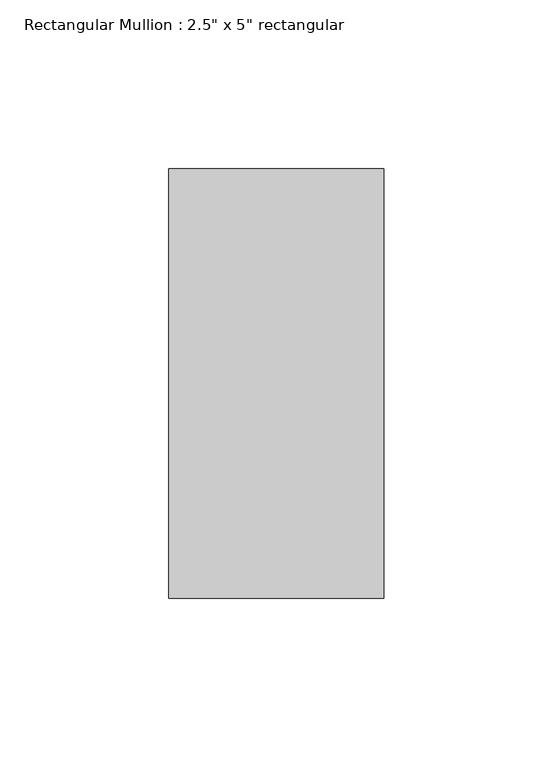
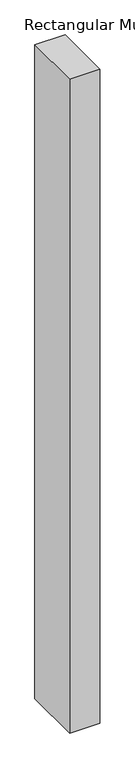
"""IFC4 building model written with IfcOpenShell, lengths in millimetres: member geometry."""

from ifc_helpers import new_model, si_unit, frame, origin, place, context, project, spatial, polyline, outline, extrude, source, transform, mapped, element, save


def member_269047fe(model_context):
    return source(origin(), model_context, "Body", "SweptSolid", [
        extrude(outline(polyline([(0.0, 63.5), (0.0, -63.5), (-63.5, -63.5), (-63.5, 63.5), (0.0, 63.5)])), frame((0.0, 0.0, -1455.9654832), z_axis=(0.0, 0.0, 1.0), x_axis=(1.0, 0.0, 0.0)), (0.0, 0.0, 1.0), 1455.9654832),
    ])


if __name__ == "__main__":
    model = new_model("IFC4")
    model_context = context("Model", 3, world=origin())
    ifc_project = project(units=[si_unit("LENGTHUNIT", "METRE", prefix="MILLI")], contexts=[model_context])
    site = spatial("IfcSite", under=ifc_project)
    building = spatial("IfcBuilding", under=site)
    placement = place(None, origin())
    member_shape = member_269047fe(model_context)
    element("IfcMember", 1, ObjectType="Rectangular Mullion : 2.5\" x 5\" rectangular", at=placement, inside=building, context=model_context, shape_type="MappedRepresentation", body=[
        mapped(member_shape, transform((0.0, 0.0, 0.0), x_axis=(1.0, 0.0, 0.0), y_axis=(0.0, 1.0, 0.0), z_axis=(0.0, 0.0, 1.0))),
    ])
    save(model, "model.ifc")

# Revit data of these elements
# Type "Rectangular Mullion : 2.5\" x 5\" rectangular"
#   built-in parameter 1007304 = 0.416667 (stored number, unit not read)
#   built-in parameter 1007301 = 0.104167 (stored number, unit not read)
#   built-in parameter 1007300 = 0.104167 (stored number, unit not read)
# Element 1 (IfcMember, "Rectangular Mullion : 2.5\" x 5\" rectangular")
#   Materials on its faces: "Aluminum"
# Materials
#   "Aluminum": class "Metal", colour RGB 247 247 247, transparency 0, Description = "Aluminum 6061", Cost = 0
